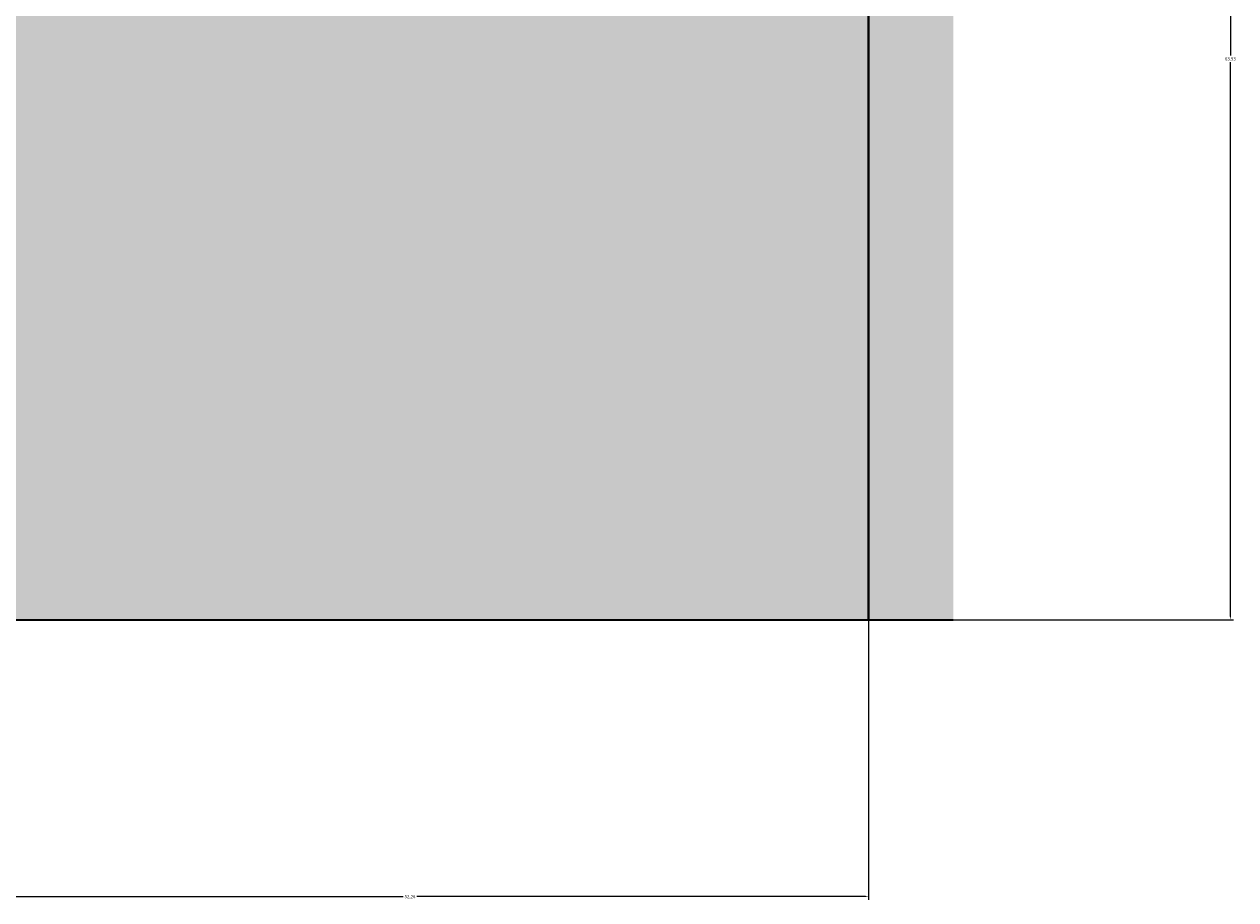
# Model space of a CAD drawing. Units: feet. Extents: x 2695 to 2912, y 795 to 1139.
# Tile 20 of 83: x 2843 to 2912, y 795 to 845. Entities that reach past the tile are written whole.
import ezdxf

# ---------------------------------------------------------------- set-up
doc = ezdxf.new("R2010")
doc.units = ezdxf.units.FT
for name, color, linetype, lineweight in [('A-ANNO-DIMS', 2, 'Continuous', 18), ('A-ELEV', 7, 'Continuous', 35), ('A-ELEV-PATT', 252, 'Continuous', 13)]:
    doc.layers.add(name, color=color, linetype=linetype, lineweight=lineweight)
doc.styles.get("Standard").update_dxf_attribs({"font": 'arial.ttf'})
doc.dimstyles.get("Standard").update_dxf_attribs({"dimtxt": 0.18, "dimasz": 0.18, "dimexe": 0.18, "dimexo": 0.0625, "dimgap": 0.09, "dimtad": 0, "dimtih": 1, "dimtoh": 1, "dimdec": 1, "dimzin": 0, "dimdsep": 46, "dimlunit": 3, "dimtxsty": 'Standard', "dimcen": 0.09, "dimadec": 0, "dimazin": 0, "dimtfac": 1, "dimtdec": 1, "dimtofl": 0, "dimtmove": 0, "dimatfit": 3, "dimfxl": 1, "dimtolj": 1, "dimtzin": 0, "dimarcsym": 0})

# ---------------------------------------------------------------- blocks, each defined once
blk = doc.blocks.new('*D6')
at = {"layer": 'A-ANNO-DIMS', "color": 0, "lineweight": -2, "transparency": 16777216}
for p, q in [((2838.377, 810.868), (2838.377, 794.976)), ((2890.636, 810.868), (2890.636, 794.976)), ((2838.557, 795.156), (2864.113, 795.156)), ((2890.456, 795.156), (2864.9, 795.156))]:
    blk.add_line(p, q, dxfattribs=at)
at = {"layer": 'A-ANNO-DIMS', "color": 0, "transparency": 16777216}
for points in [[(2838.557, 795.186), (2838.557, 795.126), (2838.377, 795.156)], [(2890.456, 795.186), (2890.456, 795.126), (2890.636, 795.156)]]:
    blk.add_solid(points, dxfattribs=at)
at = {"layer": 'Defpoints', "color": 0, "transparency": 16777216}
for p in [(2838.377, 810.931), (2890.636, 810.931), (2890.636, 795.156)]:
    blk.add_point(p, dxfattribs=at)
at = {"layer": 'A-ANNO-DIMS', "color": 0, "transparency": 16777216, "insert": (2864.506, 795.156), "char_height": 0.18, "attachment_point": 5}
blk.add_mtext('\\A1;52.26', dxfattribs=at)
blk = doc.blocks.new('*D13')
at = {"layer": 'A-ANNO-DIMS', "color": 0, "lineweight": -2, "transparency": 16777216}
for p, q in [((2758.214, 874.857), (2911.424, 874.857)), ((2911.244, 874.677), (2911.244, 843.076)), ((2911.244, 811.111), (2911.244, 842.712)), ((2890.699, 810.931), (2911.424, 810.931))]:
    blk.add_line(p, q, dxfattribs=at)
at = {"layer": 'A-ANNO-DIMS', "color": 0, "transparency": 16777216}
for points in [[(2911.214, 874.677), (2911.274, 874.677), (2911.244, 874.857)], [(2911.214, 811.111), (2911.274, 811.111), (2911.244, 810.931)]]:
    blk.add_solid(points, dxfattribs=at)
at = {"layer": 'Defpoints', "color": 0, "transparency": 16777216}
for p in [(2758.151, 874.857), (2911.244, 874.857), (2890.636, 810.931)]:
    blk.add_point(p, dxfattribs=at)
at = {"layer": 'A-ANNO-DIMS', "color": 0, "transparency": 16777216, "insert": (2911.244, 842.894), "char_height": 0.18, "attachment_point": 5}
blk.add_mtext('\\A1;63.93', dxfattribs=at)

msp = doc.modelspace()

# ---------------------------------------------------------------- hatches: boundary and pattern name
at = {"layer": 'A-ELEV-PATT'}
h = msp.add_hatch(color=256, dxfattribs=at)
h.set_gradient(color1=(147, 149, 152), color2=(147, 149, 152), tint=1)
h.paths.add_polyline_path([(2770.6361, 1118.4096), (2710.6361, 1118.4096), (2710.6361, 1062.9306), (2770.6361, 1062.9306)])
h.paths.add_polyline_path([(2890.6361, 1103.3378), (2770.6361, 1103.3378), (2770.6361, 1062.9306), (2890.6361, 1062.9306)])
h.paths.add_polyline_path([(2730.7081, 1048.1052), (2755.1125, 1048.1052), (2755.1125, 936.9306), (2770.6361, 936.9306), (2770.6361, 1050.3105), (2715.8852, 1050.3105), (2715.8852, 936.9306), (2730.7081, 936.9306)])
h.paths.add_polyline_path([(2890.6361, 1050.3105), (2770.6361, 1050.3105), (2770.6361, 971.9673), (2778.0341, 971.9673), (2778.0341, 1020.8235), (2843.575, 1020.8235), (2843.575, 971.9673), (2890.6361, 971.9673)])
h.paths.add_polyline_path([(2888.1882, 970.7156), (2843.575, 970.7156), (2843.575, 964.8267), (2888.1882, 964.8267)])
h.paths.add_polyline_path([(2888.1882, 964.1328), (2843.575, 964.1328), (2843.575, 956.614), (2888.1882, 956.614)])
h.paths.add_polyline_path([(2888.1882, 955.9202), (2843.575, 955.9202), (2843.575, 949.2892), (2888.1882, 949.2892)])
h.paths.add_polyline_path([(2888.1882, 948.5954), (2843.575, 948.5954), (2843.575, 941.3507), (2888.1882, 941.3507)])
h.paths.add_polyline_path([(2888.1882, 940.6569), (2843.575, 940.6569), (2843.575, 936.9306), (2888.1882, 936.9306)])
h.paths.add_polyline_path([(2890.6361, 970.7156), (2888.9368, 970.7156), (2888.9368, 964.8267), (2890.6361, 964.8267)])
h.paths.add_polyline_path([(2890.6361, 964.1328), (2888.9368, 964.1328), (2888.9368, 956.614), (2890.6361, 956.614)])
h.paths.add_polyline_path([(2890.6361, 955.9202), (2888.9368, 955.9202), (2888.9368, 949.2892), (2890.6361, 949.2892)])
h.paths.add_polyline_path([(2890.6361, 940.6569), (2888.9368, 940.6569), (2888.9368, 936.9306), (2890.6361, 936.9306)])
h.paths.add_polyline_path([(2890.6361, 948.5954), (2888.9368, 948.5954), (2888.9368, 941.3507), (2890.6361, 941.3507)])
h.paths.add_polyline_path([(2772.5216, 970.7156), (2770.6361, 970.7156), (2770.6361, 964.8267), (2772.5216, 964.8267)])
h.paths.add_polyline_path([(2772.5216, 964.1328), (2770.6361, 964.1328), (2770.6361, 956.614), (2772.5216, 956.614)])
h.paths.add_polyline_path([(2772.5216, 955.9202), (2770.6361, 955.9202), (2770.6361, 949.2892), (2772.5216, 949.2892)])
h.paths.add_polyline_path([(2772.5216, 948.5954), (2770.6361, 948.5954), (2770.6361, 941.3507), (2772.5216, 941.3507)])
h.paths.add_polyline_path([(2772.5216, 940.6569), (2770.6361, 940.6569), (2770.6361, 936.9306), (2772.5216, 936.9306)])
h.paths.add_polyline_path([(2778.0341, 940.6569), (2773.2702, 940.6569), (2773.2702, 936.9306), (2778.0341, 936.9306)])
h.paths.add_polyline_path([(2778.0341, 970.7156), (2773.2702, 970.7156), (2773.2702, 964.8267), (2778.0341, 964.8267)])
h.paths.add_polyline_path([(2778.0341, 964.1328), (2773.2702, 964.1328), (2773.2702, 956.614), (2778.0341, 956.614)])
h.paths.add_polyline_path([(2778.0341, 955.9202), (2773.2702, 955.9202), (2773.2702, 949.2892), (2778.0341, 949.2892)])
h.paths.add_polyline_path([(2778.0341, 948.5954), (2773.2702, 948.5954), (2773.2702, 941.3507), (2778.0341, 941.3507)])
h.paths.add_polyline_path([(2810.0407, 940.6569), (2780.0341, 940.6569), (2780.0341, 936.9306), (2810.0407, 936.9306)])
h.paths.add_polyline_path([(2890.6361, 924.3105), (2770.6361, 924.3105), (2770.6361, 810.9306), (2773.5029, 810.9306), (2773.5029, 905.5143), (2805.9398, 905.5143), (2838.3767, 905.5143), (2838.3767, 810.9306), (2890.6361, 810.9306)])
h = msp.add_hatch(color=256, dxfattribs=at)
h.set_gradient(color1=(255, 255, 255), tint=1)
h.paths.add_polyline_path([(2895.4694, 1107.8588), (2890.6361, 1107.8588), (2890.6361, 810.9306), (2895.4694, 810.9306)])

# ---------------------------------------------------------------- linework, layer by layer
at = {"layer": 'A-ELEV'}
for p, q in [((2890.6361, 810.9306), (2890.6361, 1107.8588)), ((2890.6361, 1062.9306), (2890.6361, 810.9306)), ((2710.6361, 810.9306), (2890.6361, 810.9306)), ((2710.6361, 810.9306), (2890.6361, 810.9306)), ((2710.6361, 810.9306), (2895.4426, 810.9306))]:
    msp.add_line(p, q, dxfattribs=at)

# ---------------------------------------------------------------- dimensions: what is measured, and where the dimension line sits
at = {"layer": 'A-ANNO-DIMS'}
dim = msp.add_linear_dim(base=(2911.2444, 874.8571), p1=(2890.6361, 810.9306), p2=(2758.1515, 874.8571), angle=90, dimstyle='Standard', override={"dimdec": 2, "dimlfac": 1, "dimrnd": 0, "dimzin": 0, "dimdsep": 46, "dimlunit": 2}, dxfattribs=at)
dim.commit()
dim.dimension.update_dxf_attribs({"geometry": '*D13', "text_midpoint": (2911.2444, 842.8938)})
dim = msp.add_linear_dim(base=(2890.6361, 795.1556), p1=(2838.3767, 810.9306), p2=(2890.6361, 810.9306), dimstyle='Standard', override={"dimdec": 2, "dimlfac": 1, "dimrnd": 0, "dimzin": 0, "dimdsep": 46, "dimlunit": 2}, dxfattribs=at)
dim.commit()
dim.dimension.update_dxf_attribs({"geometry": '*D6', "text_midpoint": (2864.5064, 795.1556)})

doc.saveas('drawing.dxf')
